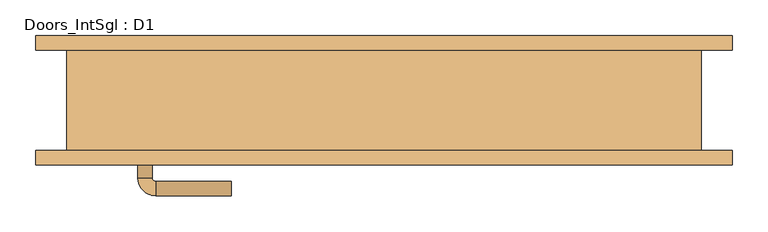
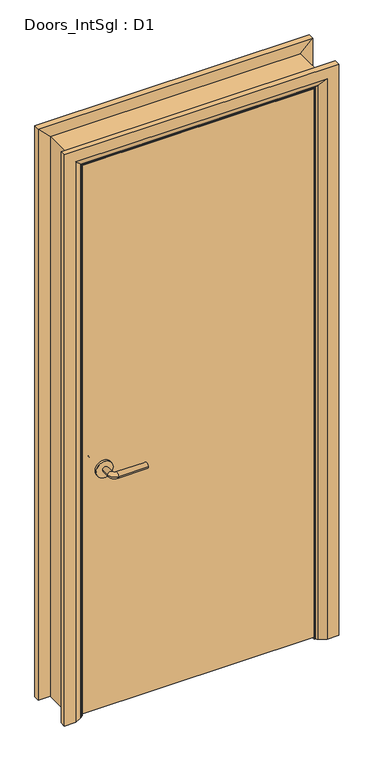
"""IFC4 building model written with IfcOpenShell, lengths in millimetres: door geometry, Doors_IntSgl : D1."""

from ifc_helpers import new_model, si_unit, point, frame, frame_2d, origin, place, context, project, spatial, polyline, circle_curve, ellipse_curve, trimmed, segment, composite_curve, outline, extrude, faceted_brep, source, transform, mapped, element, save
from ifc_brep_helpers import plane_surface, cylinder_surface, revolved_surface, advanced_brep


def doors_intsgl_d1_661c03a1(model_context):
    return source(origin(), model_context, "Body", "SolidModel", [
        advanced_brep(
        [(-343.0, -24.0, 900.0), (-323.0, -24.0, 900.0), (-343.0, 6.0, 900.0), (-323.0, 6.0, 900.0), (-318.0, 11.0, 900.0), (-318.0, 31.0, 900.0), (-213.0, 31.0, 900.0), (-213.0, 11.0, 900.0)],
        [
            (0, 1, circle_curve(frame((-333.0, -24.0, 900.0), z_axis=(0.0, -1.0, 0.0), x_axis=(1.0, 0.0, 0.0)), 10.0)),
            (1, 0, circle_curve(frame((-333.0, -24.0, 900.0), z_axis=(0.0, -1.0, 0.0), x_axis=(1.0, 0.0, 0.0)), 10.0)),
            (0, 2),
            (2, 3, circle_curve(frame((-333.0, 6.0, 900.0), z_axis=(0.0, -1.0, 0.0), x_axis=(1.0, 0.0, 0.0)), 10.0)),
            (3, 1),
            (3, 2, circle_curve(frame((-333.0, 6.0, 900.0), z_axis=(0.0, -1.0, 0.0), x_axis=(1.0, 0.0, 0.0)), 10.0)),
            (4, 3, circle_curve(frame((-318.0, 6.0, 900.0), z_axis=(0.0, 0.0, 1.0), x_axis=(-1.0, 0.0, 0.0)), 5.0)),
            (2, 5, circle_curve(frame((-318.0, 6.0, 900.0), z_axis=(0.0, 0.0, -1.0), x_axis=(-1.0, 0.0, 0.0)), 25.0)),
            (5, 4, circle_curve(frame((-318.0, 21.0, 900.0), z_axis=(-1.0, 0.0, 0.0), x_axis=(0.0, -1.0, 0.0)), 10.0)),
            (4, 5, circle_curve(frame((-318.0, 21.0, 900.0), z_axis=(-1.0, 0.0, 0.0), x_axis=(0.0, -1.0, 0.0)), 10.0)),
            (6, 7, circle_curve(frame((-213.0, 21.0, 900.0), z_axis=(1.0, 0.0, 0.0), x_axis=(0.0, -1.0, 0.0)), 10.0)),
            (7, 6, circle_curve(frame((-213.0, 21.0, 900.0), z_axis=(1.0, 0.0, 0.0), x_axis=(0.0, -1.0, 0.0)), 10.0)),
            (5, 6),
            (7, 4),
        ],
        [
            plane_surface(frame((-333.0, -24.0, 900.0), z_axis=(0.0, -1.0, 0.0), x_axis=(0.0, 0.0, 1.0))),
            cylinder_surface(frame((-333.0, -24.0, 900.0), z_axis=(0.0, -1.0, 0.0), x_axis=(1.0, 0.0, 0.0)), 10.0),
            revolved_surface(trimmed(ellipse_curve(frame((-333.0, 6.0, 900.0), z_axis=(0.0, -1.0, 0.0), x_axis=(1.0, 0.0, 0.0)), 10.0, 10.0), [point((-343.0, 6.0, 900.0))], [point((-323.0, 6.0, 900.0))], True, "CARTESIAN"), (-318.0, 6.0, 900.0), (0.0, 0.0, -1.0)),
            revolved_surface(trimmed(ellipse_curve(frame((-333.0, 6.0, 900.0), z_axis=(0.0, -1.0, 0.0), x_axis=(1.0, 0.0, 0.0)), 10.0, 10.0), [point((-323.0, 6.0, 900.0))], [point((-343.0, 6.0, 900.0))], True, "CARTESIAN"), (-318.0, 6.0, 900.0), (0.0, 0.0, -1.0)),
            plane_surface(frame((-213.0, 21.0, 900.0), z_axis=(1.0, 0.0, 0.0), x_axis=(0.0, 0.0, 1.0))),
            cylinder_surface(frame((-318.0, 21.0, 900.0), z_axis=(-1.0, 0.0, 0.0), x_axis=(0.0, -1.0, 0.0)), 10.0),
        ],
        [
            (0, [[1, 2]]),
            (1, [[-1, 3, 4, 5]]),
            (1, [[-2, -5, 6, -3]]),
            (2, [[7, -4, 8, 9]]),
            (3, [[-8, -6, -7, 10]]),
            (4, [[11, 12]]),
            (5, [[-9, 13, -12, 14]]),
            (5, [[-10, -14, -11, -13]]),
        ],
    ),
        extrude(outline(composite_curve([segment(trimmed(circle_curve(frame_2d((900.0, -335.5)), 30.0), [point((900.0, -365.5))], [point((900.0, -305.5))], False, "CARTESIAN"), True, "CONTINUOUS"), segment(trimmed(circle_curve(frame_2d((900.0, -335.5)), 30.0), [point((900.0, -305.5))], [point((900.0, -365.5))], False, "CARTESIAN"), True, "CONTINUOUS")], self_intersect=False)), frame((0.0, -32.0, 0.0), z_axis=(0.0, 1.0, 0.0), x_axis=(0.0, 0.0, 1.0)), (0.0, 0.0, 1.0), 8.0),
        advanced_brep(
        [(-343.0, -78.0, 900.0), (-323.0, -78.0, 900.0), (-323.0, -108.0, 900.0), (-343.0, -108.0, 900.0), (-318.0, -113.0, 900.0), (-318.0, -133.0, 900.0), (-213.0, -133.0, 900.0), (-213.0, -113.0, 900.0)],
        [
            (0, 1, circle_curve(frame((-333.0, -78.0, 900.0), z_axis=(0.0, 1.0, 0.0), x_axis=(1.0, 0.0, 0.0)), 10.0)),
            (1, 0, circle_curve(frame((-333.0, -78.0, 900.0), z_axis=(0.0, 1.0, 0.0), x_axis=(1.0, 0.0, 0.0)), 10.0)),
            (1, 2),
            (2, 3, circle_curve(frame((-333.0, -108.0, 900.0), z_axis=(0.0, 1.0, 0.0), x_axis=(1.0, 0.0, 0.0)), 10.0)),
            (3, 0),
            (3, 2, circle_curve(frame((-333.0, -108.0, 900.0), z_axis=(0.0, 1.0, 0.0), x_axis=(1.0, 0.0, 0.0)), 10.0)),
            (4, 5, circle_curve(frame((-318.0, -123.0, 900.0), z_axis=(-1.0, 0.0, 0.0), x_axis=(0.0, 1.0, 0.0)), 10.0)),
            (5, 3, circle_curve(frame((-318.0, -108.0, 900.0), z_axis=(0.0, 0.0, -1.0), x_axis=(-1.0, 0.0, 0.0)), 25.0)),
            (2, 4, circle_curve(frame((-318.0, -108.0, 900.0), z_axis=(0.0, 0.0, 1.0), x_axis=(-1.0, 0.0, 0.0)), 5.0)),
            (5, 4, circle_curve(frame((-318.0, -123.0, 900.0), z_axis=(-1.0, 0.0, 0.0), x_axis=(0.0, 1.0, 0.0)), 10.0)),
            (6, 7, circle_curve(frame((-213.0, -123.0, 900.0), z_axis=(1.0, 0.0, 0.0), x_axis=(0.0, 1.0, 0.0)), 10.0)),
            (7, 6, circle_curve(frame((-213.0, -123.0, 900.0), z_axis=(1.0, 0.0, 0.0), x_axis=(0.0, 1.0, 0.0)), 10.0)),
            (4, 7),
            (6, 5),
        ],
        [
            plane_surface(frame((-333.0, -78.0, 900.0), z_axis=(0.0, 1.0, 0.0), x_axis=(0.0, 0.0, 1.0))),
            cylinder_surface(frame((-333.0, -78.0, 900.0), z_axis=(0.0, 1.0, 0.0), x_axis=(1.0, 0.0, 0.0)), 10.0),
            revolved_surface(trimmed(ellipse_curve(frame((-333.0, -108.0, 900.0), z_axis=(0.0, -1.0, 0.0), x_axis=(1.0, 0.0, 0.0)), 10.0, 10.0), [point((-343.0, -108.0, 900.0))], [point((-323.0, -108.0, 900.0))], True, "CARTESIAN"), (-318.0, -108.0, 900.0), (0.0, 0.0, -1.0)),
            revolved_surface(trimmed(ellipse_curve(frame((-333.0, -108.0, 900.0), z_axis=(0.0, -1.0, 0.0), x_axis=(1.0, 0.0, 0.0)), 10.0, 10.0), [point((-323.0, -108.0, 900.0))], [point((-343.0, -108.0, 900.0))], True, "CARTESIAN"), (-318.0, -108.0, 900.0), (0.0, 0.0, -1.0)),
            plane_surface(frame((-213.0, -123.0, 900.0), z_axis=(1.0, 0.0, 0.0), x_axis=(0.0, 0.0, 1.0))),
            cylinder_surface(frame((-318.0, -123.0, 900.0), z_axis=(-1.0, 0.0, 0.0), x_axis=(0.0, 1.0, 0.0)), 10.0),
        ],
        [
            (0, [[1, 2]]),
            (1, [[3, 4, 5, -2]]),
            (1, [[-5, 6, -3, -1]]),
            (2, [[7, 8, -4, 9]]),
            (3, [[10, -9, -6, -8]]),
            (4, [[11, 12]]),
            (5, [[13, -11, 14, -7]]),
            (5, [[-14, -12, -13, -10]]),
        ],
    ),
        extrude(outline(composite_curve([segment(trimmed(circle_curve(frame_2d((900.0, -335.5)), 30.0), [point((900.0, -365.5))], [point((900.0, -305.5))], False, "CARTESIAN"), True, "CONTINUOUS"), segment(trimmed(circle_curve(frame_2d((900.0, -335.5)), 30.0), [point((900.0, -305.5))], [point((900.0, -365.5))], False, "CARTESIAN"), True, "CONTINUOUS")], self_intersect=False)), frame((0.0, -78.0, 0.0), z_axis=(0.0, 1.0, 0.0), x_axis=(0.0, 0.0, 1.0)), (0.0, 0.0, 1.0), 8.0),
        extrude(outline(polyline([(408.0, -32.0), (408.0, -70.0), (-408.0, -70.0), (-408.0, -32.0), (408.0, -32.0)])), frame((0.0, 0.0, 8.0), z_axis=(0.0, 0.0, 1.0), x_axis=(1.0, 0.0, 0.0)), (0.0, 0.0, 1.0), 2050.0),
        advanced_brep(
        [(485.0, -90.0, 0.0), (445.0, -90.0, 0.0), (419.0, -76.0, 0.0), (415.0, -70.0, 0.0), (485.0, -70.0, 0.0), (485.0, -70.0, 2135.0), (485.0, -90.0, 2135.0), (415.0, -70.0, 2065.0), (-415.0, -70.0, 2065.0), (-415.0, -70.0, 0.0), (-485.0, -70.0, 0.0), (-485.0, -70.0, 2135.0), (419.0, -76.0, 2069.0), (445.0, -90.0, 2095.0), (-485.0, -90.0, 2135.0), (-485.0, -90.0, 0.0), (-445.0, -90.0, 0.0), (-445.0, -90.0, 2095.0), (-419.0, -76.0, 0.0), (-419.0, -76.0, 2069.0)],
        [
            (0, 1),
            (1, 2),
            (2, 3, circle_curve(frame((423.0, -69.0, 0.0), z_axis=(0.0, 0.0, -1.0), x_axis=(1.0, 0.0, 0.0)), 8.0622577)),
            (3, 4),
            (4, 0),
            (4, 5),
            (5, 6),
            (6, 0),
            (3, 7),
            (7, 8),
            (8, 9),
            (9, 10),
            (10, 11),
            (11, 5),
            (2, 12),
            (12, 7, ellipse_curve(frame((423.0, -69.0, 2073.0), z_axis=(0.7071067811865475, 0.0, -0.7071067811865475), x_axis=(-0.7071067811865474, 0.0, -0.7071067811865476)), 11.4017543, 8.0622577)),
            (1, 13),
            (13, 12),
            (6, 14),
            (14, 15),
            (15, 16),
            (16, 17),
            (17, 13),
            (10, 15),
            (14, 11),
            (9, 18, circle_curve(frame((-423.0, -69.0, 0.0), z_axis=(0.0, 0.0, -1.0), x_axis=(-1.0, 0.0, 0.0)), 8.0622577)),
            (18, 16),
            (19, 18),
            (8, 19, ellipse_curve(frame((-423.0, -69.0, 2073.0), z_axis=(-0.7071067811865475, 0.0, -0.7071067811865475), x_axis=(-0.7071067811865474, 0.0, 0.7071067811865476)), 11.4017543, 8.0622577)),
            (19, 17),
            (12, 19),
        ],
        [
            plane_surface(frame((415.0, -70.0, 0.0), z_axis=(0.0, 0.0, -1.0), x_axis=(0.0, 1.0, 0.0))),
            plane_surface(frame((485.0, -90.0, 0.0), z_axis=(1.0, 0.0, 0.0), x_axis=(0.0, 0.0, 1.0))),
            plane_surface(frame((485.0, -70.0, 0.0), z_axis=(0.0, 1.0, 0.0), x_axis=(0.0, 0.0, 1.0))),
            cylinder_surface(frame((423.0, -69.0, 0.0), z_axis=(0.0, 0.0, -1.0), x_axis=(1.0, 0.0, 0.0)), 8.0622577),
            plane_surface(frame((419.0, -76.0, 0.0), z_axis=(-0.4740998230350126, -0.880471099922178, 0.0), x_axis=(0.0, 0.0, 1.0))),
            plane_surface(frame((445.0, -90.0, 0.0), z_axis=(0.0, -1.0, 0.0), x_axis=(0.0, 0.0, 1.0))),
            plane_surface(frame((-485.0, -90.0, 2135.0), z_axis=(-1.0, 0.0, 0.0), x_axis=(0.0, 0.0, -1.0))),
            plane_surface(frame((-415.0, -70.0, 0.0), z_axis=(0.0, 0.0, -1.0), x_axis=(0.0, 1.0, 0.0))),
            cylinder_surface(frame((-423.0, -69.0, 2065.0), z_axis=(0.0, 0.0, 1.0), x_axis=(-1.0, 0.0, 0.0)), 8.0622577),
            plane_surface(frame((-419.0, -76.0, 2069.0), z_axis=(0.47409982303501824, -0.8804710999221749, 0.0), x_axis=(0.0, 0.0, -1.0))),
            plane_surface(frame((485.0, -90.0, 2135.0), z_axis=(0.0, 0.0, 1.0), x_axis=(-1.0, 0.0, 0.0))),
            cylinder_surface(frame((415.0, -69.0, 2073.0), z_axis=(1.0, 0.0, 0.0), x_axis=(0.0, 0.0, 1.0)), 8.0622577),
            plane_surface(frame((419.0, -76.0, 2069.0), z_axis=(0.0, -0.8804710999221764, -0.4740998230350154), x_axis=(-1.0, 0.0, 0.0))),
        ],
        [
            (0, [[1, 2, 3, 4, 5]]),
            (1, [[6, 7, 8, -5]]),
            (2, [[9, 10, 11, 12, 13, 14, -6, -4]]),
            (3, [[15, 16, -9, -3]]),
            (4, [[17, 18, -15, -2]]),
            (5, [[-8, 19, 20, 21, 22, 23, -17, -1]]),
            (6, [[-13, 24, -20, 25]]),
            (7, [[-24, -12, 26, 27, -21]]),
            (8, [[28, -26, -11, 29]]),
            (9, [[-22, -27, -28, 30]]),
            (10, [[-14, -25, -19, -7]]),
            (11, [[31, -29, -10, -16]]),
            (12, [[-23, -30, -31, -18]]),
        ],
    ),
        extrude(outline(polyline([(0.0, -391.0), (2041.0, -391.0), (2041.0, 391.0), (0.0, 391.0), (0.0, 410.0), (2060.0, 410.0), (2060.0, -410.0), (0.0, -410.0), (0.0, -391.0)])), frame((0.0, -30.0, 0.0), z_axis=(0.0, 1.0, 0.0), x_axis=(0.0, 0.0, 1.0)), (0.0, 0.0, 1.0), 32.0),
        advanced_brep(
        [(-485.0, 90.0, 0.0), (-445.0, 90.0, 0.0), (-419.0, 76.0, 0.0), (-415.0, 70.0, 0.0), (-485.0, 70.0, 0.0), (-485.0, 70.0, 2135.0), (-485.0, 90.0, 2135.0), (-415.0, 70.0, 2065.0), (-419.0, 76.0, 2069.0), (-445.0, 90.0, 2095.0), (485.0, 90.0, 0.0), (485.0, 70.0, 0.0), (415.0, 70.0, 0.0), (419.0, 76.0, 0.0), (445.0, 90.0, 0.0), (485.0, 90.0, 2135.0), (445.0, 90.0, 2095.0), (419.0, 76.0, 2069.0), (415.0, 70.0, 2065.0), (485.0, 70.0, 2135.0)],
        [
            (0, 1),
            (1, 2),
            (2, 3, circle_curve(frame((-423.0, 69.0, 0.0), z_axis=(0.0, 0.0, -1.0), x_axis=(-1.0, 0.0, 0.0)), 8.0622577)),
            (3, 4),
            (4, 0),
            (4, 5),
            (5, 6),
            (6, 0),
            (3, 7),
            (7, 5),
            (2, 8),
            (8, 7, ellipse_curve(frame((-423.0, 69.0, 2073.0), z_axis=(-0.7071067811865475, 0.0, -0.7071067811865475), x_axis=(0.7071067811865474, 0.0, -0.7071067811865476)), 11.4017543, 8.0622577)),
            (1, 9),
            (9, 8),
            (6, 9),
            (10, 11),
            (11, 12),
            (12, 13, circle_curve(frame((423.0, 69.0, 0.0), z_axis=(0.0, 0.0, -1.0), x_axis=(1.0, 0.0, 0.0)), 8.0622577)),
            (13, 14),
            (14, 10),
            (15, 10),
            (14, 16),
            (16, 15),
            (13, 17),
            (17, 16),
            (12, 18),
            (18, 17, ellipse_curve(frame((423.0, 69.0, 2073.0), z_axis=(0.7071067811865475, 0.0, -0.7071067811865475), x_axis=(0.7071067811865474, 0.0, 0.7071067811865476)), 11.4017543, 8.0622577)),
            (11, 19),
            (19, 18),
            (15, 19),
            (5, 19),
            (15, 6),
            (7, 18),
            (8, 17),
            (9, 16),
        ],
        [
            plane_surface(frame((-415.0, 142.8010989, 0.0), z_axis=(0.0, 0.0, -1.0), x_axis=(1.0, 0.0, 0.0))),
            plane_surface(frame((-485.0, 90.0, 0.0), z_axis=(-1.0, 0.0, 0.0), x_axis=(0.0, 0.0, 1.0))),
            plane_surface(frame((-485.0, 70.0, 0.0), z_axis=(0.0, -1.0, 0.0), x_axis=(0.0, 0.0, 1.0))),
            cylinder_surface(frame((-423.0, 69.0, 0.0), z_axis=(0.0, 0.0, -1.0), x_axis=(-1.0, 0.0, 0.0)), 8.0622577),
            plane_surface(frame((-419.0, 76.0, 0.0), z_axis=(0.4740998230350183, 0.8804710999221749, 0.0), x_axis=(0.0, 0.0, 1.0))),
            plane_surface(frame((-445.0, 90.0, 0.0), z_axis=(0.0, 1.0, 0.0), x_axis=(0.0, 0.0, 1.0))),
            plane_surface(frame((415.0, 142.8010989, 0.0), z_axis=(0.0, 0.0, -1.0), x_axis=(-1.0, 0.0, 0.0))),
            plane_surface(frame((445.0, 90.0, 2095.0), z_axis=(0.0, 1.0, 0.0), x_axis=(0.0, 0.0, -1.0))),
            plane_surface(frame((419.0, 76.0, 2069.0), z_axis=(-0.4740998230350183, 0.8804710999221749, 0.0), x_axis=(0.0, 0.0, -1.0))),
            cylinder_surface(frame((423.0, 69.0, 2065.0), z_axis=(0.0, 0.0, 1.0), x_axis=(1.0, 0.0, 0.0)), 8.0622577),
            plane_surface(frame((485.0, 70.0, 2135.0), z_axis=(0.0, -1.0, 0.0), x_axis=(0.0, 0.0, -1.0))),
            plane_surface(frame((485.0, 90.0, 2135.0), z_axis=(1.0, 0.0, 0.0), x_axis=(0.0, 0.0, -1.0))),
            plane_surface(frame((-485.0, 90.0, 2135.0), z_axis=(0.0, 0.0, 1.0), x_axis=(1.0, 0.0, 0.0))),
            plane_surface(frame((-485.0, 70.0, 2135.0), z_axis=(0.0, -1.0, 0.0), x_axis=(1.0, 0.0, 0.0))),
            cylinder_surface(frame((-415.0, 69.0, 2073.0), z_axis=(-1.0, 0.0, 0.0), x_axis=(0.0, 0.0, 1.0)), 8.0622577),
            plane_surface(frame((-419.0, 76.0, 2069.0), z_axis=(0.0, 0.8804710999221749, -0.4740998230350183), x_axis=(1.0, 0.0, 0.0))),
            plane_surface(frame((-445.0, 90.0, 2095.0), z_axis=(0.0, 1.0, 0.0), x_axis=(1.0, 0.0, 0.0))),
        ],
        [
            (0, [[1, 2, 3, 4, 5]]),
            (1, [[6, 7, 8, -5]]),
            (2, [[9, 10, -6, -4]]),
            (3, [[11, 12, -9, -3]]),
            (4, [[13, 14, -11, -2]]),
            (5, [[-8, 15, -13, -1]]),
            (6, [[16, 17, 18, 19, 20]]),
            (7, [[21, -20, 22, 23]]),
            (8, [[-22, -19, 24, 25]]),
            (9, [[-24, -18, 26, 27]]),
            (10, [[-26, -17, 28, 29]]),
            (11, [[-28, -16, -21, 30]]),
            (12, [[31, -30, 32, -7]]),
            (13, [[33, -29, -31, -10]]),
            (14, [[34, -27, -33, -12]]),
            (15, [[35, -25, -34, -14]]),
            (16, [[-32, -23, -35, -15]]),
        ],
    ),
        faceted_brep([(-410.0, -70.0, 0.0), (-442.0, -70.0, 0.0), (-442.0, 70.0, 0.0), (-410.0, 70.0, 0.0), (-410.0, 70.0, 2060.0), (-410.0, -70.0, 2060.0), (-442.0, 70.0, 2092.0), (-442.0, -70.0, 2092.0), (410.0, -70.0, 0.0), (410.0, 70.0, 0.0), (442.0, 70.0, 0.0), (442.0, -70.0, 0.0), (410.0, -70.0, 2060.0), (442.0, -70.0, 2092.0), (442.0, 70.0, 2092.0), (410.0, 70.0, 2060.0)], [[[0, 1, 2, 3]], [[3, 4, 5, 0]], [[2, 6, 4, 3]], [[1, 7, 6, 2]], [[0, 5, 7, 1]], [[8, 9, 10, 11]], [[12, 8, 11, 13]], [[13, 11, 10, 14]], [[14, 10, 9, 15]], [[15, 9, 8, 12]], [[4, 15, 12, 5]], [[6, 14, 15, 4]], [[7, 13, 14, 6]], [[5, 12, 13, 7]]]),
    ])


if __name__ == "__main__":
    model = new_model("IFC4")
    model_context = context("Model", 3, world=origin())
    ifc_project = project(units=[si_unit("LENGTHUNIT", "METRE", prefix="MILLI")], contexts=[model_context])
    site = spatial("IfcSite", under=ifc_project)
    building = spatial("IfcBuilding", under=site)
    placement = place(None, origin())
    doors_intsgl_d1_shape = doors_intsgl_d1_661c03a1(model_context)
    element("IfcDoor", 1, ObjectType="Doors_IntSgl : D1", at=placement, inside=building, context=model_context, shape_type="MappedRepresentation", body=[
        mapped(doors_intsgl_d1_shape, transform((0.0, 0.0, 0.0), x_axis=(1.0, 0.0, 0.0), y_axis=(0.0, 1.0, 0.0), z_axis=(0.0, 0.0, 1.0))),
    ])
    save(model, "model.ifc")

# Revit data of these elements
# Type "Doors_IntSgl : D1"
#   Type Mark = "46"
#   Type Comments = "Internal Single"
#   Operation = "SingleSwingRight"
#   Manufacturer = "Revit"
#   Keynote = "L20"
#   Description = "Internal Single Door"
#   Analytic Construction = "Metal"
#   UnderCut = 8 mm
#   Tolerance = 2 mm
#   Thickness = 38 mm
#   Thermal Resistance (R) = 0.270117 (m²·K)/W
#   Structural Tolerance = 8 mm
#   StopDepth = 32 mm
#   Stop Thickness = 19 mm
#   Rough Width = 900 mm
#   Rough Height = 2100 mm
#   Height to Top Lock Rail = 1000 mm
#   Heat Transfer Coefficient (U) = 3.7021 W/(m²·K)
#   Handle Z Distance = 900 mm
#   Handle X Distance = 75 mm
#   Frame Thickness = 32 mm
#   Door Panel Width = 816 mm
#   Door Panel Thickness = 38 mm
#   Door Panel Offset = 0 mm
#   Height = 2100 mm
#   Width = 900 mm
#   Door Panel Height = 2050 mm
#   Architrave Setback = 5 mm
#   Vis - Ironmongery = yes
#   Material Ironmongery = Door - Handle
#   Material Frame = Door - Frame/Mullion (1)
#   Material Door = Door - Panel
#   Material Architrave = Door - Architrave
#   Visual Light Transmittance = 0
#   Solar Heat Gain Coefficient = 0
#   Function = (empty or 0)
#   Wall Closure = (empty or 0)
# Element 1 (IfcDoor, "Doors_IntSgl : D1")
#   Materials on its faces: "Door - Architrave", "Door - Handle", "Door - Frame/Mullion (1)", "Door - Panel"
# Materials
#   "Door - Handle": colour RGB 0 0 0, transparency 0, Keynote = "P21", Cost = 0
#   "Door - Frame/Mullion (1)": class "Wood", colour RGB 212 179 113, transparency 0, Keynote = "L20", Cost = 0
#   "Door - Panel": class "Wood", colour RGB 210 159 95, transparency 0, Keynote = "L20", Cost = 0
#   "Door - Architrave": class "Wood", colour RGB 154 90 5, transparency 0, Keynote = "P20", Cost = 0
